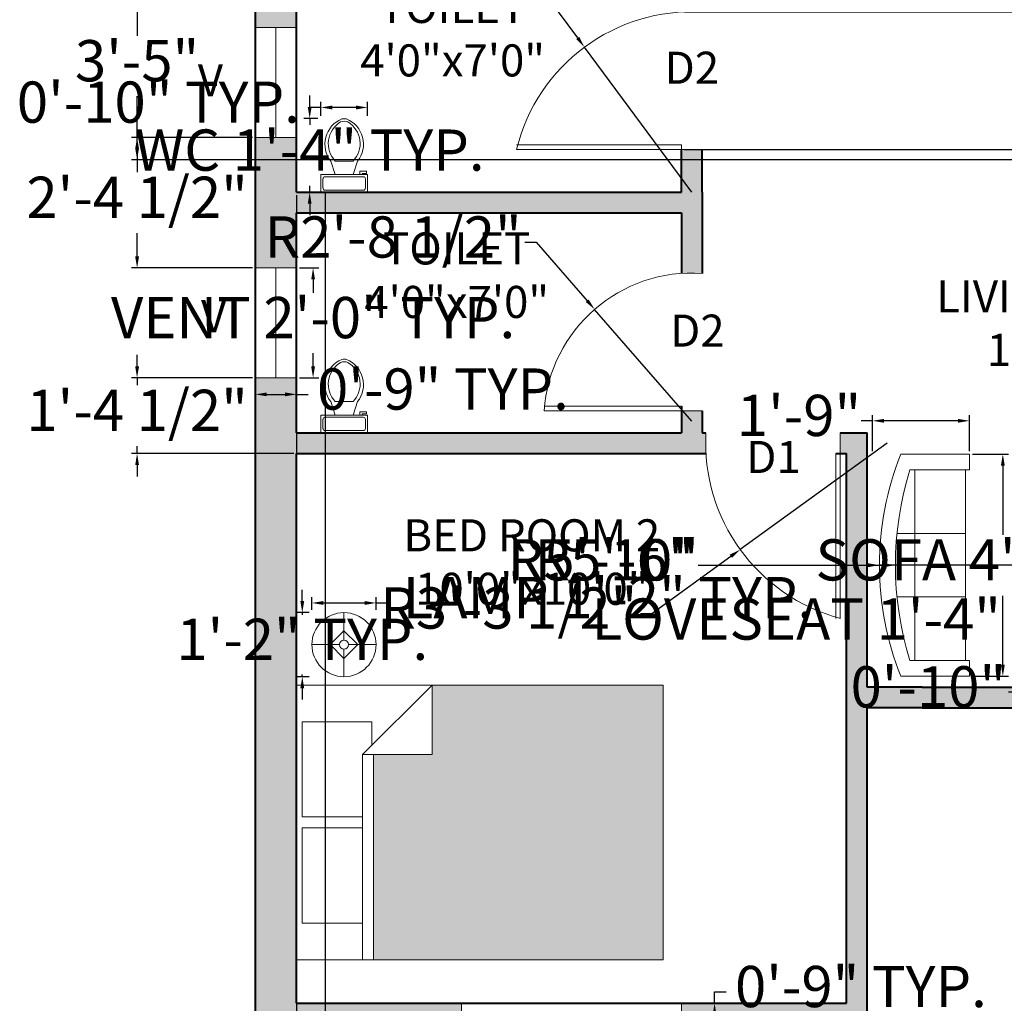
# Model space of a CAD drawing. Units: inches. Extents: x 1883 to 2353, y 1976 to 2541.
# Tile 2 of 5: x 1955 to 2170, y 2132 to 2346. Entities that reach past the tile are written whole.
import ezdxf

# ---------------------------------------------------------------- set-up
doc = ezdxf.new("R2010")
doc.units = ezdxf.units.IN
for name, color, linetype, lineweight in [('A-ANNO-DIMS', 2, 'Continuous', 18), ('A-ANNO-TEXT', 7, 'Continuous', 18), ('A-AREA-IDEN', 7, 'Continuous', 18), ('A-DOOR', 3, 'Continuous', 18), ('A-FLOR-FIXT', 9, 'Continuous', 18), ('A-FURN', 8, 'Continuous', 18), ('A-GLAZ', 4, 'Continuous', 18), ('A-WALL', 7, 'Continuous', 40)]:
    doc.layers.add(name, color=color, linetype=linetype, lineweight=lineweight)
doc.layers.add('A-FURN-PATT', color=18, linetype='Continuous', lineweight=13, true_color=0x000000)
doc.layers.add('A-WALL-PATT', color=67, linetype='Continuous', lineweight=13, true_color=0x727430)
doc.styles.get("Standard").update_dxf_attribs({"font": 'arial.ttf'})
doc.dimstyles.new('ISO-25', dxfattribs={"dimtxt": 9, "dimasz": 2.5, "dimexe": 1.25, "dimexo": 0.625, "dimgap": 2, "dimtad": 0, "dimtih": 1, "dimtoh": 1, "dimdec": 1, "dimlunit": 4, "dimtxsty": 'Standard', "dimcen": 2.5, "dimadec": 0, "dimazin": 0, "dimtfac": 1, "dimtdec": 1, "dimtmove": 0, "dimatfit": 3, "dimfxl": 1, "dimarcsym": 0})

# ---------------------------------------------------------------- blocks, each defined once
blk = doc.blocks.new('Toilet - top')
for p, q in [((9.5, -6), (9.5, -2)), ((-10, -8.5), (-8, -8.5)), ((-10, -9.5), (-10, -8.5)), ((-8, -8.5), (-8, -8)), ((-7, -8), (-7, -9.5)), ((-4, -8), (-6, -14)), ((4, -8), (6, -14)), ((-7, -9.5), (-10, -9.5)), ((4, -14), (-4, -14))]:
    blk.add_line(p, q)
blk.add_lwpolyline([(10.5, -8), (10.5, 0), (-10.5, 0), (-10.5, -8)], close=True)
for points in [[(-9.5, -2), (-9.5, -6)], [(8.5, -1), (-8.5, -1)], [(-8.5, -7), (8.5, -7)]]:
    blk.add_lwpolyline(points)
for centre, radius, start, end in [((-8.62, -1.88), 0.884, 81.8699, 188.1301), ((8.62, -1.88), 0.884, 351.8699, 98.1301), ((-8.62, -6.12), 0.884, 171.8699, 278.1301), ((8.62, -6.12), 0.884, 261.8699, 8.1301), ((3.52, -21.58), 12.17, 141.4691, 247.9714), ((4.2, -21.82), 11.33, 136.3677, 238.9468), ((-3.52, -21.58), 12.17, 292.0284, 38.5307), ((-4.2, -21.82), 11.33, 301.053, 43.6321), ((0, -27.88), 4, 245.7318, 294.2682), ((0, -29), 4, 254.8605, 285.1395)]:
    blk.add_arc(centre, radius, start, end)
blk = doc.blocks.new('Bed - Queen')
for p, q in [((0, -80.00003), (0, 0)), ((0, 0), (59.99999, 0)), ((59.99999, 0), (59.99999, -80.00003)), ((7.99999, -1.2), (28.79998, -1.2)), ((7.99999, -14.4), (7.99999, -1.2)), ((28.79998, -1.2), (28.79998, -14.4)), ((31.19999, -1.2), (51.99999, -1.2)), ((31.19999, -14.4), (31.19999, -1.2)), ((51.99999, -1.2), (51.99999, -16.4)), ((0, -14.4), (44.8, -14.4)), ((59.99999, -29.6), (44.8, -14.4)), ((44.8, -14.4), (44.8, -29.6)), ((44.8, -16.8), (0, -16.8)), ((51.99999, -16.4), (46.79936, -16.4)), ((44.8, -29.6), (59.99999, -29.6)), ((59.99999, -80.00003), (0, -80.00003))]:
    blk.add_line(p, q)
blk = doc.blocks.new('Sofa - Roundback 7 ft.')
for p, q in [((-12.00002, -32.4421), (-12.00003, -6.5971)), ((11.99997, -32.4421), (11.99998, -6.5971)), ((-36.000027, -34), (-36.000027, -11.4696)), ((-35.999844, -13.3819), (35.9998, -13.3819)), ((35.99998, -34), (35.99998, -11.4696)), ((-36.000027, -32.4421), (35.99998, -32.4421))]:
    blk.add_line(p, q)
for points in [[(-36.000027, -34), (-42.000027, -34), (-42.000027, -8)], [(41.99998, -8), (41.99998, -34), (35.99998, -34)]]:
    blk.add_lwpolyline(points)
for centre, radius, start, end in [((0, -114.25), 114.25, 68.43141, 111.5686), ((-0.00001, -127.1968), 121.1968, 72.72033, 107.2797)]:
    blk.add_arc(centre, radius, start, end)
blk = doc.blocks.new('Lamp - Table')
for p, q in [((0, 7), (0, 1)), ((0, 3), (-3, 0)), ((3, 0), (0, 3)), ((-1, 0), (-7, 0)), ((-3, 0), (0, -3)), ((0, -3), (3, 0)), ((1, 0), (7, 0)), ((0, -1), (0, -7))]:
    blk.add_line(p, q)
for radius in [7, 1]:
    blk.add_circle((0, 0), radius)
blk = doc.blocks.new('WIN-48IN')
for p, q in [((0, 0), (0, 9)), ((48, 0), (48, 9)), ((0, 4.5), (48, 4.5))]:
    blk.add_line(p, q)
blk = doc.blocks.new('VENT-24IN')
for p, q in [((9, 24), (0, 24)), ((4.5, 24), (4.5, 0)), ((9, 0), (0, 0))]:
    blk.add_line(p, q)
blk = doc.blocks.new('*D19')
at = {"layer": 'A-ANNO-DIMS', "color": 0, "lineweight": -2, "transparency": 16777216}
for p, q in [((2018.83, 2217.48), (2018.83, 2220.2)), ((2032.83, 2217.48), (2032.83, 2220.2)), ((2021.33, 2218.95), (2030.33, 2218.95)), ((2032.83, 2218.95), (2035.33, 2218.95))]:
    blk.add_line(p, q, dxfattribs=at)
at = {"layer": 'A-ANNO-DIMS', "color": 0, "transparency": 16777216}
for points in [[(2021.33, 2219.37), (2021.33, 2218.53), (2018.83, 2218.95)], [(2030.33, 2219.37), (2030.33, 2218.53), (2032.83, 2218.95)]]:
    blk.add_solid(points, dxfattribs=at)
at = {"layer": 'Defpoints', "color": 0, "transparency": 16777216}
for p in [(2032.83, 2218.95), (2018.83, 2216.85), (2032.83, 2216.85)]:
    blk.add_point(p, dxfattribs=at)
at = {"layer": 'A-ANNO-DIMS', "color": 0, "transparency": 16777216, "insert": (2083.43, 2218.95), "char_height": 9, "attachment_point": 5}
blk.add_mtext('LAMP 1\'-2" TYP.', dxfattribs=at)
blk = doc.blocks.new('*D20')
at = {"layer": 'A-ANNO-DIMS', "color": 0, "lineweight": -2, "transparency": 16777216}
for p, q in [((2016.73, 2219.35), (2016.73, 2221.85)), ((2018.2, 2216.85), (2015.48, 2216.85)), ((2016.73, 2216.85), (2016.73, 2216.37)), ((2018.2, 2202.85), (2015.48, 2202.85)), ((2016.73, 2202.85), (2016.73, 2203.33)), ((2016.73, 2200.35), (2016.73, 2197.85))]:
    blk.add_line(p, q, dxfattribs=at)
at = {"layer": 'A-ANNO-DIMS', "color": 0, "transparency": 16777216}
for points in [[(2016.31, 2219.35), (2017.15, 2219.35), (2016.73, 2216.85)], [(2016.31, 2200.35), (2017.15, 2200.35), (2016.73, 2202.85)]]:
    blk.add_solid(points, dxfattribs=at)
at = {"layer": 'Defpoints', "color": 0, "transparency": 16777216}
for p in [(2016.73, 2216.85), (2018.83, 2216.85), (2018.83, 2202.85)]:
    blk.add_point(p, dxfattribs=at)
at = {"layer": 'A-ANNO-DIMS', "color": 0, "transparency": 16777216, "insert": (2016.73, 2209.85), "char_height": 9, "attachment_point": 5}
blk.add_mtext('1\'-2" TYP.', dxfattribs=at)
blk = doc.blocks.new('*D21')
at = {"layer": 'A-ANNO-DIMS', "color": 0, "lineweight": -2, "transparency": 16777216}
for p, q in [((2051.49, 2121.95), (2051.49, 2114.12)), ((2099.49, 2121.95), (2099.49, 2114.12)), ((2053.99, 2115.37), (2096.99, 2115.37)), ((2099.49, 2115.37), (2101.99, 2115.37))]:
    blk.add_line(p, q, dxfattribs=at)
at = {"layer": 'A-ANNO-DIMS', "color": 0, "transparency": 16777216}
for points in [[(2053.99, 2115.79), (2053.99, 2114.96), (2051.49, 2115.37)], [(2096.99, 2115.79), (2096.99, 2114.96), (2099.49, 2115.37)]]:
    blk.add_solid(points, dxfattribs=at)
at = {"layer": 'Defpoints', "color": 0, "transparency": 16777216}
for p in [(2051.49, 2122.57), (2099.49, 2122.57), (2099.49, 2115.37)]:
    blk.add_point(p, dxfattribs=at)
at = {"layer": 'A-ANNO-DIMS', "color": 0, "transparency": 16777216, "insert": (2160.94, 2115.37), "char_height": 9, "attachment_point": 5}
blk.add_mtext('WINDOW 4\'-0" TYP.', dxfattribs=at)
blk = doc.blocks.new('*D22')
at = {"layer": 'A-ANNO-DIMS', "color": 0, "lineweight": -2, "transparency": 16777216}
for p, q in [((2106.69, 2131.57), (2106.69, 2134.07)), ((2106.69, 2134.07), (2109.19, 2134.07)), ((2100.12, 2131.57), (2107.94, 2131.57)), ((2106.69, 2125.07), (2106.69, 2129.07)), ((2100.12, 2122.57), (2107.94, 2122.57))]:
    blk.add_line(p, q, dxfattribs=at)
at = {"layer": 'A-ANNO-DIMS', "color": 0, "transparency": 16777216}
for points in [[(2106.28, 2129.07), (2107.11, 2129.07), (2106.69, 2131.57)], [(2106.28, 2125.07), (2107.11, 2125.07), (2106.69, 2122.57)]]:
    blk.add_solid(points, dxfattribs=at)
at = {"layer": 'Defpoints', "color": 0, "transparency": 16777216}
for p in [(2099.49, 2131.57), (2106.69, 2131.57), (2099.49, 2122.57)]:
    blk.add_point(p, dxfattribs=at)
at = {"layer": 'A-ANNO-DIMS', "color": 0, "transparency": 16777216, "insert": (2138.62, 2134.07), "char_height": 9, "attachment_point": 5}
blk.add_mtext('0\'-9" TYP.', dxfattribs=at)
blk = doc.blocks.new('*D23')
at = {"layer": 'A-ANNO-DIMS', "color": 0, "lineweight": -2, "transparency": 16777216}
for p, q in [((2018.35, 2327.17), (2018.35, 2329.67)), ((2020.13, 2324.67), (2017.1, 2324.67)), ((2018.35, 2324.67), (2018.35, 2323.27)), ((2018.35, 2308.57), (2018.35, 2309.97)), ((2020.13, 2308.57), (2017.1, 2308.57)), ((2018.35, 2306.07), (2018.35, 2303.57))]:
    blk.add_line(p, q, dxfattribs=at)
at = {"layer": 'A-ANNO-DIMS', "color": 0, "transparency": 16777216}
for points in [[(2017.93, 2327.17), (2018.76, 2327.17), (2018.35, 2324.67)], [(2017.93, 2306.07), (2018.76, 2306.07), (2018.35, 2308.57)]]:
    blk.add_solid(points, dxfattribs=at)
at = {"layer": 'Defpoints', "color": 0, "transparency": 16777216}
for p in [(2020.76, 2324.67), (2018.35, 2308.57), (2020.76, 2308.57)]:
    blk.add_point(p, dxfattribs=at)
at = {"layer": 'A-ANNO-DIMS', "color": 0, "transparency": 16777216, "insert": (2018.35, 2316.62), "char_height": 9, "attachment_point": 5}
blk.add_mtext('WC 1\'-4" TYP.', dxfattribs=at)
blk = doc.blocks.new('*D24')
at = {"layer": 'A-ANNO-DIMS', "color": 0, "lineweight": -2, "transparency": 16777216}
for p, q in [((2020.76, 2327.09), (2018.26, 2327.09)), ((2020.76, 2325.3), (2020.76, 2328.34)), ((2028.49, 2327.09), (2023.26, 2327.09)), ((2030.99, 2325.3), (2030.99, 2328.34))]:
    blk.add_line(p, q, dxfattribs=at)
at = {"layer": 'A-ANNO-DIMS', "color": 0, "transparency": 16777216}
for points in [[(2023.26, 2327.5), (2023.26, 2326.67), (2020.76, 2327.09)], [(2028.49, 2327.5), (2028.49, 2326.67), (2030.99, 2327.09)]]:
    blk.add_solid(points, dxfattribs=at)
at = {"layer": 'Defpoints', "color": 0, "transparency": 16777216}
for p in [(2020.76, 2327.09), (2020.76, 2324.67), (2030.99, 2324.67)]:
    blk.add_point(p, dxfattribs=at)
at = {"layer": 'A-ANNO-DIMS', "color": 0, "transparency": 16777216, "insert": (1985.33, 2327.09), "char_height": 9, "attachment_point": 5}
blk.add_mtext('0\'-10" TYP.', dxfattribs=at)
blk = doc.blocks.new('*D27')
at = {"layer": 'A-ANNO-DIMS', "color": 0, "lineweight": -2, "transparency": 16777216}
for p, q in [((2016.12, 2292.07), (2020.34, 2292.07)), ((2019.09, 2289.57), (2019.09, 2286.67)), ((2019.09, 2270.57), (2019.09, 2273.48)), ((2016.12, 2268.07), (2020.34, 2268.07))]:
    blk.add_line(p, q, dxfattribs=at)
at = {"layer": 'A-ANNO-DIMS', "color": 0, "transparency": 16777216}
for points in [[(2018.68, 2289.57), (2019.51, 2289.57), (2019.09, 2292.07)], [(2018.68, 2270.57), (2019.51, 2270.57), (2019.09, 2268.07)]]:
    blk.add_solid(points, dxfattribs=at)
at = {"layer": 'Defpoints', "color": 0, "transparency": 16777216}
for p in [(2015.49, 2292.07), (2019.09, 2292.07), (2015.49, 2268.07)]:
    blk.add_point(p, dxfattribs=at)
at = {"layer": 'A-ANNO-DIMS', "color": 0, "transparency": 16777216, "insert": (2019.09, 2280.07), "char_height": 9, "attachment_point": 5}
blk.add_mtext('VENT 2\'-0" TYP.', dxfattribs=at)
blk = doc.blocks.new('*D28')
at = {"layer": 'A-ANNO-DIMS', "color": 0, "lineweight": -2, "transparency": 16777216}
for p, q in [((2006.49, 2267.45), (2006.49, 2263.22)), ((2015.49, 2267.45), (2015.49, 2263.22)), ((2008.99, 2264.47), (2012.99, 2264.47)), ((2015.49, 2264.47), (2017.99, 2264.47))]:
    blk.add_line(p, q, dxfattribs=at)
at = {"layer": 'A-ANNO-DIMS', "color": 0, "transparency": 16777216}
for points in [[(2008.99, 2264.89), (2008.99, 2264.06), (2006.49, 2264.47)], [(2012.99, 2264.89), (2012.99, 2264.06), (2015.49, 2264.47)]]:
    blk.add_solid(points, dxfattribs=at)
at = {"layer": 'Defpoints', "color": 0, "transparency": 16777216}
for p in [(2006.49, 2268.07), (2015.49, 2268.07), (2015.49, 2264.47)]:
    blk.add_point(p, dxfattribs=at)
at = {"layer": 'A-ANNO-DIMS', "color": 0, "transparency": 16777216, "insert": (2047.42, 2264.47), "char_height": 9, "attachment_point": 5}
blk.add_mtext('0\'-9" TYP.', dxfattribs=at)
blk = doc.blocks.new('*D33')
at = {"layer": 'A-ANNO-DIMS', "color": 0, "lineweight": -2, "transparency": 16777216}
for p, q in [((2162.94, 2251.43), (2170.84, 2251.43)), ((2169.59, 2248.93), (2169.59, 2233.85)), ((2169.59, 2205.45), (2169.59, 2220.53)), ((2162.94, 2202.95), (2170.84, 2202.95))]:
    blk.add_line(p, q, dxfattribs=at)
at = {"layer": 'A-ANNO-DIMS', "color": 0, "transparency": 16777216}
for points in [[(2169.17, 2248.93), (2170.01, 2248.93), (2169.59, 2251.43)], [(2169.17, 2205.45), (2170.01, 2205.45), (2169.59, 2202.95)]]:
    blk.add_solid(points, dxfattribs=at)
at = {"layer": 'Defpoints', "color": 0, "transparency": 16777216}
for p in [(2162.32, 2251.43), (2169.59, 2251.43), (2162.32, 2202.95)]:
    blk.add_point(p, dxfattribs=at)
at = {"layer": 'A-ANNO-DIMS', "color": 0, "transparency": 16777216, "insert": (2169.59, 2227.19), "char_height": 9, "attachment_point": 5}
blk.add_mtext('SOFA 4\'-0 1/2"', dxfattribs=at)
blk = doc.blocks.new('*D34')
at = {"layer": 'A-ANNO-DIMS', "color": 0, "lineweight": -2, "transparency": 16777216}
for p, q in [((2141.15, 2258.71), (2138.65, 2258.71)), ((2141.15, 2252.06), (2141.15, 2259.96)), ((2159.82, 2258.71), (2143.65, 2258.71)), ((2162.32, 2252.06), (2162.32, 2259.96))]:
    blk.add_line(p, q, dxfattribs=at)
at = {"layer": 'A-ANNO-DIMS', "color": 0, "transparency": 16777216}
for points in [[(2143.65, 2259.12), (2143.65, 2258.29), (2141.15, 2258.71)], [(2159.82, 2259.12), (2159.82, 2258.29), (2162.32, 2258.71)]]:
    blk.add_solid(points, dxfattribs=at)
at = {"layer": 'Defpoints', "color": 0, "transparency": 16777216}
for p in [(2141.15, 2258.71), (2141.15, 2251.43), (2162.32, 2251.43)]:
    blk.add_point(p, dxfattribs=at)
at = {"layer": 'A-ANNO-DIMS', "color": 0, "transparency": 16777216, "insert": (2125.12, 2258.71), "char_height": 9, "attachment_point": 5}
blk.add_mtext('1\'-9"', dxfattribs=at)
blk = doc.blocks.new('*D35')
at = {"layer": 'A-ANNO-DIMS', "color": 0, "lineweight": -2, "transparency": 16777216}
for p, q in [((2175.72, 2212.47), (2175.72, 2215.52)), ((2191.87, 2212.47), (2191.87, 2215.52)), ((2175.72, 2214.27), (2173.22, 2214.27)), ((2189.37, 2214.27), (2178.22, 2214.27))]:
    blk.add_line(p, q, dxfattribs=at)
at = {"layer": 'A-ANNO-DIMS', "color": 0, "transparency": 16777216}
for points in [[(2178.22, 2214.69), (2178.22, 2213.85), (2175.72, 2214.27)], [(2189.37, 2214.69), (2189.37, 2213.85), (2191.87, 2214.27)]]:
    blk.add_solid(points, dxfattribs=at)
at = {"layer": 'Defpoints', "color": 0, "transparency": 16777216}
for p in [(2175.72, 2214.27), (2175.72, 2211.85), (2191.87, 2211.85)]:
    blk.add_point(p, dxfattribs=at)
at = {"layer": 'A-ANNO-DIMS', "color": 0, "transparency": 16777216, "insert": (2124.52, 2214.27), "char_height": 9, "attachment_point": 5}
blk.add_mtext('LOVESEAT 1\'-4"', dxfattribs=at)
blk = doc.blocks.new('*D36')
at = {"layer": 'A-ANNO-DIMS', "color": 0, "lineweight": -2, "transparency": 16777216}
for p, q in [((2175.1, 2211.85), (2172.05, 2211.85)), ((2173.3, 2209.35), (2173.3, 2204.48)), ((2175.1, 2201.98), (2172.05, 2201.98)), ((2173.3, 2201.98), (2173.3, 2199.48)), ((2173.3, 2199.48), (2170.8, 2199.48))]:
    blk.add_line(p, q, dxfattribs=at)
at = {"layer": 'A-ANNO-DIMS', "color": 0, "transparency": 16777216}
for points in [[(2172.88, 2209.35), (2173.72, 2209.35), (2173.3, 2211.85)], [(2172.88, 2204.48), (2173.72, 2204.48), (2173.3, 2201.98)]]:
    blk.add_solid(points, dxfattribs=at)
at = {"layer": 'Defpoints', "color": 0, "transparency": 16777216}
for p in [(2175.72, 2211.85), (2173.3, 2201.98), (2175.72, 2201.98)]:
    blk.add_point(p, dxfattribs=at)
at = {"layer": 'A-ANNO-DIMS', "color": 0, "transparency": 16777216, "insert": (2153.34, 2199.48), "char_height": 9, "attachment_point": 5}
blk.add_mtext('0\'-10"', dxfattribs=at)
blk = doc.blocks.new('*D48')
at = {"layer": 'A-ANNO-DIMS', "color": 0, "lineweight": -2, "transparency": 16777216}
for p, q in [((2260.87, 2356.57), (1979.44, 2356.57)), ((1980.69, 2354.07), (1980.69, 2342.73)), ((1980.69, 2318.19), (1980.69, 2329.53)), ((2260.87, 2315.69), (1979.44, 2315.69))]:
    blk.add_line(p, q, dxfattribs=at)
at = {"layer": 'A-ANNO-DIMS', "color": 0, "transparency": 16777216}
for points in [[(1980.28, 2354.07), (1981.11, 2354.07), (1980.69, 2356.57)], [(1980.28, 2318.19), (1981.11, 2318.19), (1980.69, 2315.69)]]:
    blk.add_solid(points, dxfattribs=at)
at = {"layer": 'Defpoints', "color": 0, "transparency": 16777216}
for p in [(1980.69, 2356.57), (2261.49, 2356.57), (2261.49, 2315.69)]:
    blk.add_point(p, dxfattribs=at)
at = {"layer": 'A-ANNO-DIMS', "color": 0, "transparency": 16777216, "insert": (1980.69, 2336.13), "char_height": 9, "attachment_point": 5}
blk.add_mtext('3\'-5"', dxfattribs=at)
blk = doc.blocks.new('*D54')
at = {"layer": 'A-ANNO-DIMS', "color": 0, "lineweight": -2, "transparency": 16777216}
for p, q in [((2100.12, 2347.93), (2301.39, 2347.93)), ((2300.14, 2345.43), (2300.14, 2339.52)), ((2300.14, 2320.43), (2300.14, 2326.33)), ((2100.12, 2317.93), (2301.39, 2317.93))]:
    blk.add_line(p, q, dxfattribs=at)
at = {"layer": 'A-ANNO-DIMS', "color": 0, "transparency": 16777216}
for points in [[(2299.73, 2345.43), (2300.56, 2345.43), (2300.14, 2347.93)], [(2299.73, 2320.43), (2300.56, 2320.43), (2300.14, 2317.93)]]:
    blk.add_solid(points, dxfattribs=at)
at = {"layer": 'Defpoints', "color": 0, "transparency": 16777216}
for p in [(2099.49, 2347.93), (2300.14, 2347.93), (2099.49, 2317.93)]:
    blk.add_point(p, dxfattribs=at)
at = {"layer": 'A-ANNO-DIMS', "color": 0, "transparency": 16777216, "insert": (2300.14, 2332.93), "char_height": 9, "attachment_point": 5}
blk.add_mtext('2\'-6"', dxfattribs=at)
blk = doc.blocks.new('*D55')
at = {"layer": 'A-ANNO-DIMS', "color": 0, "lineweight": -2, "transparency": 16777216}
for p, q in [((1980.69, 2270.57), (1980.69, 2273.07)), ((2005.87, 2268.07), (1979.44, 2268.07)), ((1980.69, 2268.07), (1980.69, 2266.48)), ((2014.87, 2251.57), (1979.44, 2251.57)), ((1980.69, 2251.57), (1980.69, 2253.17)), ((1980.69, 2249.07), (1980.69, 2246.57))]:
    blk.add_line(p, q, dxfattribs=at)
at = {"layer": 'A-ANNO-DIMS', "color": 0, "transparency": 16777216}
for points in [[(1980.28, 2270.57), (1981.11, 2270.57), (1980.69, 2268.07)], [(1980.28, 2249.07), (1981.11, 2249.07), (1980.69, 2251.57)]]:
    blk.add_solid(points, dxfattribs=at)
at = {"layer": 'Defpoints', "color": 0, "transparency": 16777216}
for p in [(2006.49, 2268.07), (1980.69, 2251.57), (2015.49, 2251.57)]:
    blk.add_point(p, dxfattribs=at)
at = {"layer": 'A-ANNO-DIMS', "color": 0, "transparency": 16777216, "insert": (1980.69, 2259.82), "char_height": 9, "attachment_point": 5}
blk.add_mtext('1\'-4 1/2"', dxfattribs=at)
blk = doc.blocks.new('*D56')
at = {"layer": 'A-ANNO-DIMS', "color": 0, "lineweight": -2, "transparency": 16777216}
for p, q in [((2005.87, 2320.57), (1979.44, 2320.57)), ((1980.69, 2318.07), (1980.69, 2312.98)), ((1980.69, 2294.57), (1980.69, 2299.67)), ((2005.87, 2292.07), (1979.44, 2292.07))]:
    blk.add_line(p, q, dxfattribs=at)
at = {"layer": 'A-ANNO-DIMS', "color": 0, "transparency": 16777216}
for points in [[(1980.28, 2318.07), (1981.11, 2318.07), (1980.69, 2320.57)], [(1980.28, 2294.57), (1981.11, 2294.57), (1980.69, 2292.07)]]:
    blk.add_solid(points, dxfattribs=at)
at = {"layer": 'Defpoints', "color": 0, "transparency": 16777216}
for p in [(1980.69, 2320.57), (2006.49, 2320.57), (2006.49, 2292.07)]:
    blk.add_point(p, dxfattribs=at)
at = {"layer": 'A-ANNO-DIMS', "color": 0, "transparency": 16777216, "insert": (1980.69, 2306.32), "char_height": 9, "attachment_point": 5}
blk.add_mtext('2\'-4 1/2"', dxfattribs=at)
blk = doc.blocks.new('*D57')
at = {"layer": 'A-ANNO-DIMS', "color": 0, "lineweight": -2, "transparency": 16777216}
for p, q in [((2015.49, 2307.95), (2015.49, 1987.78)), ((2021.73, 2308.43), (2021.73, 1987.78)), ((2012.99, 1989.03), (2010.49, 1989.03)), ((2015.49, 1989.03), (2021.73, 1989.03)), ((2024.23, 1989.03), (2026.73, 1989.03))]:
    blk.add_line(p, q, dxfattribs=at)
at = {"layer": 'A-ANNO-DIMS', "color": 0, "transparency": 16777216}
for points in [[(2012.99, 1989.45), (2012.99, 1988.61), (2015.49, 1989.03)], [(2024.23, 1989.45), (2024.23, 1988.61), (2021.73, 1989.03)]]:
    blk.add_solid(points, dxfattribs=at)
at = {"layer": 'Defpoints', "color": 0, "transparency": 16777216}
for p in [(2015.49, 2308.57), (2021.73, 2309.06), (2021.73, 1989.03)]:
    blk.add_point(p, dxfattribs=at)
at = {"layer": 'A-ANNO-DIMS', "color": 0, "transparency": 16777216, "insert": (2040.7, 1989.03), "char_height": 9, "attachment_point": 5}
blk.add_mtext('0\'-6"', dxfattribs=at)
blk = doc.blocks.new('*D59')
at = {"layer": 'A-ANNO-DIMS', "color": 0, "lineweight": -2, "transparency": 16777216}
for p, q in [((2144.34, 2253.82), (2112.27, 2230.61)), ((2093.03, 2216.68), (2110.24, 2229.14)), ((2090.53, 2216.68), (2093.03, 2216.68))]:
    blk.add_line(p, q, dxfattribs=at)
at = {"layer": 'A-ANNO-DIMS', "color": 0, "transparency": 16777216}
blk.add_solid([(2110, 2229.48), (2110.49, 2228.8), (2112.27, 2230.61)], dxfattribs=at)
at = {"layer": 'Defpoints', "color": 0, "transparency": 16777216}
for p in [(2144.34, 2253.82), (2112.27, 2230.61)]:
    blk.add_point(p, dxfattribs=at)
at = {"layer": 'A-ANNO-DIMS', "color": 0, "transparency": 16777216, "insert": (2061.78, 2216.68), "char_height": 9, "attachment_point": 5}
blk.add_mtext('R3\'-3 1/2"', dxfattribs=at)
blk = doc.blocks.new('*D60')
at = {"layer": 'A-ANNO-DIMS', "color": 0, "lineweight": -2, "transparency": 16777216}
for p, q in [((2061.75, 2359.24), (2064.25, 2359.24)), ((2064.25, 2359.24), (2076.82, 2342.27)), ((2101.74, 2308.63), (2078.31, 2340.26))]:
    blk.add_line(p, q, dxfattribs=at)
at = {"layer": 'A-ANNO-DIMS', "color": 0, "transparency": 16777216}
blk.add_solid([(2077.16, 2342.51), (2076.49, 2342.02), (2078.31, 2340.26)], dxfattribs=at)
at = {"layer": 'Defpoints', "color": 0, "transparency": 16777216}
for p in [(2078.31, 2340.26), (2101.74, 2308.63)]:
    blk.add_point(p, dxfattribs=at)
at = {"layer": 'A-ANNO-DIMS', "color": 0, "transparency": 16777216, "insert": (2033, 2359.24), "char_height": 9, "attachment_point": 5}
blk.add_mtext('R3\'-3 1/2"', dxfattribs=at)
blk = doc.blocks.new('*D62')
at = {"layer": 'A-ANNO-DIMS', "color": 0, "lineweight": -2, "transparency": 16777216}
for p, q in [((2065.3, 2297.66), (2067.8, 2297.66)), ((2067.8, 2297.66), (2078.89, 2284.91)), ((2101.74, 2258.63), (2080.53, 2283.03))]:
    blk.add_line(p, q, dxfattribs=at)
at = {"layer": 'A-ANNO-DIMS', "color": 0, "transparency": 16777216}
blk.add_solid([(2079.2, 2285.19), (2078.58, 2284.64), (2080.53, 2283.03)], dxfattribs=at)
at = {"layer": 'Defpoints', "color": 0, "transparency": 16777216}
for p in [(2080.53, 2283.03), (2101.74, 2258.63)]:
    blk.add_point(p, dxfattribs=at)
at = {"layer": 'A-ANNO-DIMS', "color": 0, "transparency": 16777216, "insert": (2036.55, 2297.66), "char_height": 9, "attachment_point": 5}
blk.add_mtext('R2\'-8 1/2"', dxfattribs=at)
blk = doc.blocks.new('*D64')
at = {"layer": 'A-ANNO-DIMS', "color": 0, "lineweight": -2, "transparency": 16777216}
for p, q in [((2104.18, 2227.19), (2143.66, 2227.19)), ((2216.11, 2227.19), (2146.16, 2227.19))]:
    blk.add_line(p, q, dxfattribs=at)
at = {"layer": 'A-ANNO-DIMS', "color": 0, "transparency": 16777216}
blk.add_solid([(2143.66, 2227.61), (2143.66, 2226.77), (2146.16, 2227.19)], dxfattribs=at)
at = {"layer": 'Defpoints', "color": 0, "transparency": 16777216}
for p in [(2146.16, 2227.19), (2216.11, 2227.19)]:
    blk.add_point(p, dxfattribs=at)
at = {"layer": 'A-ANNO-DIMS', "color": 0, "transparency": 16777216, "insert": (2082.42, 2227.19), "char_height": 9, "attachment_point": 5}
blk.add_mtext('R5\'-10"', dxfattribs=at)
blk = doc.blocks.new('*D65')
at = {"layer": 'A-ANNO-DIMS', "color": 0, "lineweight": -2, "transparency": 16777216}
for p, q in [((2103.13, 2227.19), (2140.19, 2227.19)), ((2208.64, 2227.19), (2142.69, 2227.19))]:
    blk.add_line(p, q, dxfattribs=at)
at = {"layer": 'A-ANNO-DIMS', "color": 0, "transparency": 16777216}
blk.add_solid([(2140.19, 2227.61), (2140.19, 2226.77), (2142.69, 2227.19)], dxfattribs=at)
at = {"layer": 'Defpoints', "color": 0, "transparency": 16777216}
for p in [(2142.69, 2227.19), (2208.64, 2227.19)]:
    blk.add_point(p, dxfattribs=at)
at = {"layer": 'A-ANNO-DIMS', "color": 0, "transparency": 16777216, "insert": (2084.86, 2227.19), "char_height": 9, "attachment_point": 5}
blk.add_mtext('R5\'-6"', dxfattribs=at)

msp = doc.modelspace()

# ---------------------------------------------------------------- hatches: boundary and pattern name
at = {"layer": 'A-FURN-PATT'}
h = msp.add_hatch(color=256, dxfattribs=at)
h.dxf.hatch_style = 1
h.paths.add_polyline_path([(2095.49, 2464.74), (2045.09, 2464.74), (2045.09, 2449.54), (2032.29, 2449.54), (2032.29, 2404.74), (2095.49, 2404.74)])
h.paths.add_polyline_path([(2095.49, 2201.04), (2045.09, 2201.04), (2045.09, 2185.84), (2032.29, 2185.84), (2032.29, 2141.04), (2095.49, 2141.04)])
at = {"layer": 'A-WALL-PATT'}
h = msp.add_hatch(color=256, dxfattribs=at)
h.dxf.hatch_style = 1
h.paths.add_polyline_path([(2057.49, 2502.07), (2006.49, 2502.07), (2006.49, 2344.57), (2015.49, 2344.57), (2015.49, 2356.57), (2099.49, 2356.57), (2099.49, 2347.93), (2103.99, 2347.93), (2103.99, 2356.57), (2108.06, 2356.57, -0.029386), (2108.06, 2361.07), (2015.49, 2361.07), (2015.49, 2493.07), (2057.49, 2493.07)])
h.paths.add_polyline_path([(2182.74, 2502.07), (2105.49, 2502.07), (2105.49, 2493.07), (2147.49, 2493.07), (2147.49, 2361.07), (2144.06, 2361.07), (2144.06, 2356.57), (2151.99, 2356.57), (2155, 2356.57), (2155, 2361.07), (2151.99, 2361.07), (2151.99, 2493.07), (2182.74, 2493.07)])
h.paths.add_polyline_path([(2270.49, 2502.07), (2230.74, 2502.07), (2230.74, 2493.07), (2261.49, 2493.07), (2261.49, 2361.07), (2191, 2361.07, -0.029386), (2191, 2356.57), (2261.49, 2356.57), (2261.49, 2315.69), (2270.49, 2315.69)])
h.paths.add_polyline_path([(2051.49, 2131.57), (2015.49, 2131.57), (2015.49, 2251.57), (2103.99, 2251.57), (2104.81, 2251.57, -0.028441), (2104.81, 2256.07), (2103.99, 2256.07), (2103.99, 2260.88), (2099.49, 2260.88), (2099.49, 2256.07), (2015.49, 2256.07), (2015.49, 2268.07), (2006.49, 2268.07), (2006.49, 2122.57), (2015.49, 2122.57), (2051.49, 2122.57)])
h.paths.add_polyline_path([(2103.99, 2308.57), (2103.99, 2317.93, -0.034841), (2099.49, 2317.93), (2099.49, 2308.57), (2015.49, 2308.57), (2015.49, 2320.57), (2006.49, 2320.57), (2006.49, 2292.07), (2015.49, 2292.07), (2015.49, 2304.07), (2099.49, 2304.07), (2099.49, 2290.88, -0.034841), (2103.99, 2290.88), (2103.99, 2304.07)])
h = msp.add_hatch(color=256, dxfattribs=at)
h.dxf.hatch_style = 1
h.paths.add_polyline_path([(2189.49, 2090.74), (2180.49, 2090.74), (2180.49, 2071.57, -0.034524), (2180.49, 2067.07), (2189.49, 2067.07), (2261.49, 2067.07), (2270.49, 2067.07), (2270.49, 2094.07), (2270.49, 2255.69), (2261.49, 2255.69), (2261.49, 2200.57), (2261.49, 2196.07), (2261.49, 2094.07), (2261.49, 2076.07), (2189.49, 2076.07)])
h.paths.add_polyline_path([(2189.49, 2196.07), (2208.94, 2196.07), (2208.94, 2200.57), (2151.99, 2200.57), (2139.99, 2200.57), (2139.99, 2251.57), (2139.99, 2256.07), (2135.49, 2256.07), (2134.13, 2256.07), (2134.13, 2251.57), (2135.49, 2251.57), (2135.49, 2131.57), (2099.49, 2131.57), (2099.49, 2122.57), (2103.99, 2122.57), (2135.49, 2122.57), (2139.99, 2122.57), (2139.99, 2196.07), (2151.99, 2196.07), (2180.49, 2196.07), (2180.49, 2136.51), (2189.49, 2136.51)])

# ---------------------------------------------------------------- linework, layer by layer
at = {"layer": 'A-DOOR'}
for p, q in [((2099.49, 2318.93), (2063.49, 2318.93)), ((2099.49, 2317.93), (2099.49, 2318.93)), ((2099.49, 2317.93), (2063.49, 2317.93)), ((2099.49, 2317.93), (2103.99, 2317.93)), ((2099.49, 2261.88), (2069.49, 2261.88)), ((2099.49, 2260.88), (2069.49, 2260.88)), ((2099.49, 2260.88), (2103.99, 2260.88)), ((2134.13, 2251.57), (2134.13, 2256.07)), ((2133.13, 2251.57), (2133.13, 2215.57)), ((2134.13, 2251.57), (2134.13, 2215.57))]:
    msp.add_line(p, q, dxfattribs=at)
for centre, radius, start, end in [((2101.74, 2308.63), 39.36, 86.7233, 166.3344), ((2101.74, 2258.63), 32.33, 86.0091, 176.0091), ((2144.34, 2253.82), 39.59, 176.7417, 255.0672)]:
    msp.add_arc(centre, radius, start, end, dxfattribs=at)
at = {"layer": 'A-WALL'}
for p, q in [((2006.49, 2122.57), (2006.49, 2502.07)), ((2015.49, 2308.57), (2015.49, 2356.57)), ((2099.49, 2308.57), (2099.49, 2317.93)), ((2103.99, 2308.57), (2103.99, 2317.93)), ((2015.49, 2308.57), (2099.49, 2308.57)), ((2103.99, 2308.57), (2103.99, 2304.07)), ((2015.49, 2304.07), (2099.49, 2304.07)), ((2015.49, 2256.07), (2015.49, 2304.07)), ((2099.49, 2304.07), (2099.49, 2290.88)), ((2103.99, 2304.07), (2103.99, 2290.88)), ((2099.49, 2261.88), (2099.49, 2256.07)), ((2103.99, 2260.88), (2103.99, 2256.07)), ((2015.49, 2256.07), (2099.49, 2256.07)), ((2103.99, 2256.07), (2104.81, 2256.07)), ((2134.13, 2256.07), (2135.49, 2256.07)), ((2135.49, 2256.07), (2139.99, 2256.07)), ((2139.99, 2251.57), (2139.99, 2256.07)), ((2015.49, 2251.57), (2103.99, 2251.57)), ((2015.49, 2131.57), (2015.49, 2251.57)), ((2103.99, 2251.57), (2104.81, 2251.57)), ((2133.13, 2251.57), (2135.49, 2251.57)), ((2135.49, 2131.57), (2135.49, 2251.57)), ((2139.99, 2200.57), (2139.99, 2251.57)), ((2151.99, 2200.57), (2139.99, 2200.57)), ((2151.99, 2200.57), (2208.94, 2200.57)), ((2139.99, 2122.57), (2139.99, 2196.07)), ((2151.99, 2196.07), (2139.99, 2196.07)), ((2151.99, 2196.07), (2180.49, 2196.07)), ((2015.49, 2131.57), (2103.99, 2131.57)), ((2015.49, 2131.57), (2135.49, 2131.57)), ((2103.99, 2131.57), (2135.49, 2131.57))]:
    msp.add_line(p, q, dxfattribs=at)

# ---------------------------------------------------------------- block references
at = {"layer": 'A-FLOR-FIXT', "xscale": 0.4871589834253886, "yscale": 0.4871589834253886, "zscale": 0.4871589834253886, "rotation": 180}
for p in [(2025.88, 2308.57), (2025.88, 2256.07)]:
    msp.add_blockref('Toilet - top', p, dxfattribs=at)
at = {"layer": 'A-FURN', "xscale": 0.5771961655226049, "yscale": 0.5771961655226049, "zscale": 0.5771961655226049, "rotation": 90}
msp.add_blockref('Sofa - Roundback 7 ft.', (2142.69, 2227.19), dxfattribs=at)
at = {"layer": 'A-FURN'}
msp.add_blockref('Lamp - Table', (2025.83, 2209.85), dxfattribs=at)
at = {"layer": 'A-FURN', "rotation": 90}
msp.add_blockref('Bed - Queen', (2015.49, 2141.04), dxfattribs=at)
at = {"layer": 'A-GLAZ'}
for name, p in [('VENT-24IN', (2006.49, 2320.57)), ('VENT-24IN', (2006.49, 2268.07)), ('WIN-48IN', (2051.49, 2122.57))]:
    msp.add_blockref(name, p, dxfattribs=at)

# ---------------------------------------------------------------- texts
at = {"layer": 'A-ANNO-TEXT', "char_height": 7, "attachment_point": 1}
for s, width, insert in [('\\pxqc;{\\fArial|b1|i0|c0|p34;D2}', 8.1444, (2097.67, 2339.26)), ('\\pxqc;{\\fArial|b1|i0|c0|p34;V}', 12.2802, (1990.54, 2336.51)), ('\\pxqc;{\\fArial|b1|i0|c0|p34;V}', 12.2802, (1991.26, 2285.04)), ('\\pxqc;{\\fArial|b1|i0|c0|p34;D2}', 8.1444, (2098.87, 2281.89)), ('\\pxqc;{\\fArial|b1|i0|c0|p34;D1}', 15.7077, (2111.7, 2254.31))]:
    msp.add_mtext_dynamic_manual_height_columns(s, width=width, gutter_width=12.5, heights=[0], dxfattribs=dict(at, insert=insert))
at = {"layer": 'A-AREA-IDEN', "char_height": 7, "attachment_point": 1}
for s, width, insert in [('\\pxqc;{\\fArial|b1|i0|c0|p34;TOILET\\P4\'0"x7\'0"}', 65.0789, (2017, 2352.53)), ('\\pxqc;{\\fArial|b1|i0|c0|p34;TOILET\\P4\'0"x7\'0"}', 65.0789, (2017.89, 2299.82)), ('\\pxqc;{\\fArial|b1|i0|c0|p34;LIVING/DINNING\\P11\'0"x13\'0"}', 79.6787, (2151.7, 2289.36)), ('\\pxqc;{\\fArial|b1|i0|c0|p34;BED ROOM 2\\P10\'0"x10\'0"}', 71.9372, (2030.85, 2237.21))]:
    msp.add_mtext_dynamic_manual_height_columns(s, width=width, gutter_width=12.5, heights=[0], dxfattribs=dict(at, insert=insert))

# ---------------------------------------------------------------- dimensions: what is measured, and where the dimension line sits
at = {"layer": 'A-ANNO-DIMS'}
for center, mpoint, picture, middle in [((2101.74, 2308.63), (2078.31, 2340.26), '*D60', (2033, 2359.24)), ((2101.74, 2258.63), (2080.53, 2283.03), '*D62', (2036.55, 2297.66)), ((2144.34, 2253.82), (2112.27, 2230.61), '*D59', (2061.78, 2216.68)), ((2216.1109, 2227.1903), (2146.1566, 2227.19), '*D64', (2104.184, 2227.1898)), ((2208.6381, 2227.1903), (2142.6934, 2227.19), '*D65', (2103.1266, 2227.1898))]:
    dim = msp.add_radius_dim(center=center, mpoint=mpoint, dimstyle='ISO-25', override={"dimdec": 1, "dimlfac": 1, "dimrnd": 0, "dimzin": 1, "dimdsep": 46, "dimlunit": 4, "dimfrac": 2}, dxfattribs=at)
    dim.commit()
    dim.dimension.update_dxf_attribs({"geometry": picture, "text_midpoint": middle, "dimtype": 164})
for base, p1, p2, angle, picture, middle in [((1980.69, 2356.57), (2261.49, 2315.69), (2261.49, 2356.57), 90, '*D48', (1980.69, 2336.13)), ((2300.14, 2347.93), (2099.49, 2317.93), (2099.49, 2347.93), 90, '*D54', (2300.14, 2332.93)), ((1980.69, 2320.57), (2006.49, 2292.07), (2006.49, 2320.57), 90, '*D56', (1980.69, 2306.32)), ((1980.69, 2251.57), (2006.49, 2268.07), (2015.49, 2251.57), 90, '*D55', (1980.69, 2259.82)), ((2141.15, 2258.71), (2162.32, 2251.43), (2141.15, 2251.43), 180, '*D34', (2125.12, 2258.71)), ((2173.3, 2201.98), (2175.72, 2211.85), (2175.72, 2201.98), 270, '*D36', (2153.34, 2199.48))]:
    dim = msp.add_linear_dim(base=base, p1=p1, p2=p2, angle=angle, dimstyle='ISO-25', override={"dimdec": 1, "dimlfac": 1, "dimrnd": 0, "dimzin": 1, "dimdsep": 46, "dimlunit": 4, "dimfrac": 2}, dxfattribs=at)
    dim.commit()
    dim.dimension.update_dxf_attribs({"geometry": picture, "text_midpoint": middle})
for base, p1, p2, angle, text, picture, middle in [((2020.76, 2327.09), (2030.99, 2324.67), (2020.76, 2324.67), 180, '<> TYP.', '*D24', (1985.33, 2327.09)), ((2018.35, 2308.57), (2020.76, 2324.67), (2020.76, 2308.57), 270, 'WC <> TYP.', '*D23', (2018.35, 2316.62)), ((2019.09, 2292.07), (2015.49, 2268.07), (2015.49, 2292.07), 90, 'VENT <> TYP.', '*D27', (2019.09, 2280.07)), ((2169.59, 2251.43), (2162.32, 2202.95), (2162.32, 2251.43), 90, 'SOFA <>', '*D33', (2169.59, 2227.19)), ((2175.7232, 2214.2703), (2191.8719, 2211.848), (2175.7232, 2211.848), 180, 'LOVESEAT <>', '*D35', (2124.5227, 2214.2703)), ((2016.73, 2216.85), (2018.83, 2202.85), (2018.83, 2216.85), 90, '<> TYP.', '*D20', (2016.73, 2209.85)), ((2106.69, 2131.57), (2099.49, 2122.57), (2099.49, 2131.57), 90, '<> TYP.', '*D22', (2138.62, 2134.07))]:
    dim = msp.add_linear_dim(base=base, p1=p1, p2=p2, angle=angle, text=text, dimstyle='ISO-25', override={"dimdec": 1, "dimlfac": 1, "dimrnd": 0, "dimzin": 1, "dimdsep": 46, "dimlunit": 4, "dimfrac": 2}, dxfattribs=at)
    dim.commit()
    dim.dimension.update_dxf_attribs({"geometry": picture, "text_midpoint": middle})
dim = msp.add_linear_dim(base=(2021.73, 1989.03), p1=(2015.49, 2308.57), p2=(2021.73, 2309.06), dimstyle='ISO-25', override={"dimdec": 1, "dimlfac": 1, "dimrnd": 0, "dimzin": 1, "dimdsep": 46, "dimlunit": 4, "dimfrac": 2}, dxfattribs=at)
dim.commit()
dim.dimension.update_dxf_attribs({"geometry": '*D57', "text_midpoint": (2040.7, 1989.03)})
for base, p1, p2, text, picture, middle in [((2015.49, 2264.47), (2006.49, 2268.07), (2015.49, 2268.07), '<> TYP.', '*D28', (2047.42, 2264.47)), ((2032.83, 2218.95), (2018.83, 2216.85), (2032.83, 2216.85), 'LAMP <> TYP.', '*D19', (2083.43, 2218.95)), ((2099.49, 2115.37), (2051.49, 2122.57), (2099.49, 2122.57), 'WINDOW <> TYP.', '*D21', (2160.94, 2115.37))]:
    dim = msp.add_linear_dim(base=base, p1=p1, p2=p2, text=text, dimstyle='ISO-25', override={"dimdec": 1, "dimlfac": 1, "dimrnd": 0, "dimzin": 1, "dimdsep": 46, "dimlunit": 4, "dimfrac": 2}, dxfattribs=at)
    dim.commit()
    dim.dimension.update_dxf_attribs({"geometry": picture, "text_midpoint": middle})

doc.saveas('drawing.dxf')
